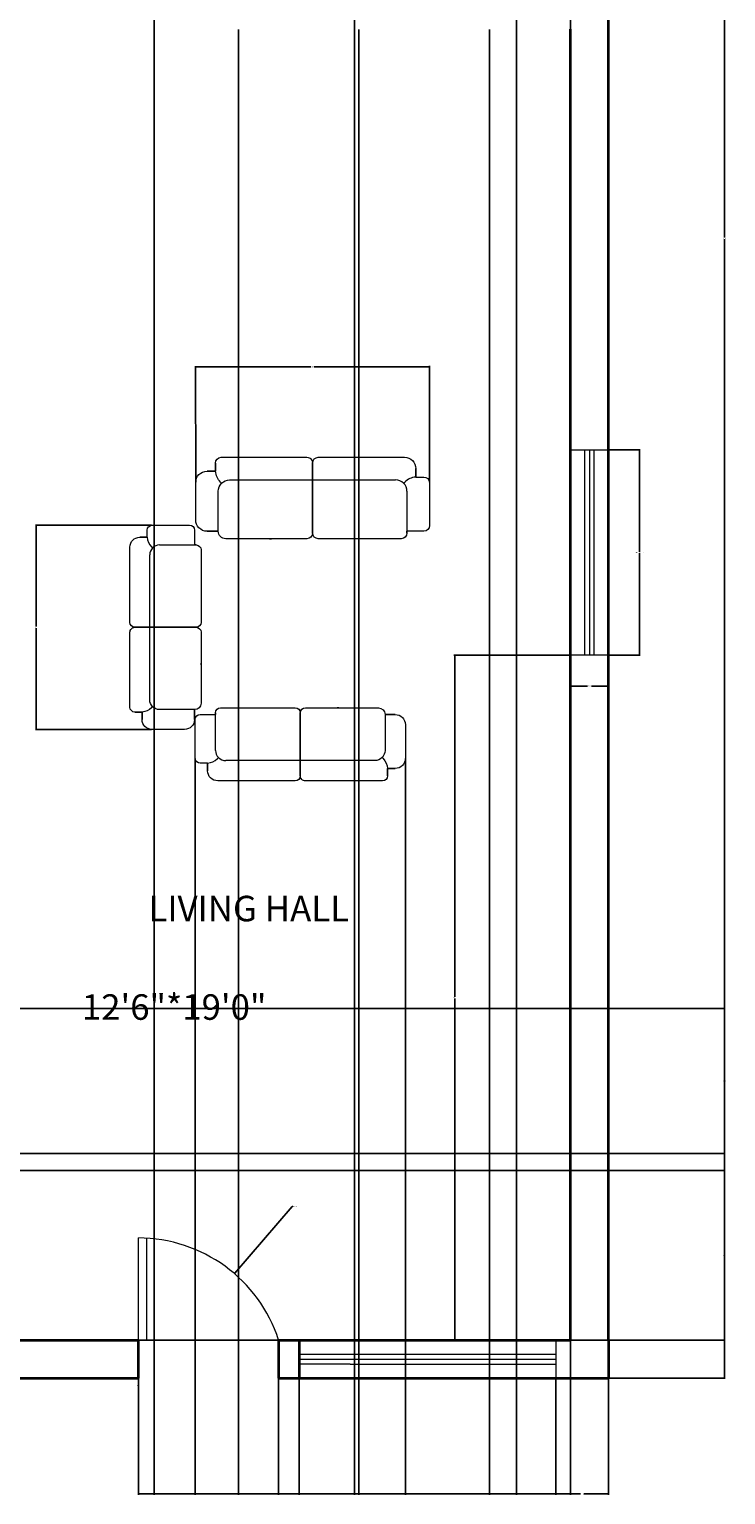
# Model space of a CAD drawing. Units: inches. Extents: x -17 to 1735, y -531 to 60.
# Tile 2 of 27: x 193 to 357, y -531 to -187. Entities that reach past the tile are written whole.
import ezdxf

# ---------------------------------------------------------------- set-up
doc = ezdxf.new("R2010")
doc.units = ezdxf.units.IN
doc.header["$MEASUREMENT"] = 0
for name, color, linetype, lineweight in [('A-ANNO-DIMS', 2, 'Continuous', 18), ('A-AREA-IDEN', 7, 'Continuous', 25), ('A-DOOR', 4, 'Continuous', 18), ('A-GLAZ', 4, 'Continuous', 18), ('A-WALL', 7, 'Continuous', 35)]:
    doc.layers.add(name, color=color, linetype=linetype, lineweight=lineweight)
doc.layers.add('A-FURN', color=242, linetype='Continuous', lineweight=18, true_color=0xcd2027)
doc.styles.get("Standard").update_dxf_attribs({"font": 'arial.ttf'})
doc.dimstyles.get("Standard").update_dxf_attribs({"dimtxt": 0.18, "dimasz": 0.18, "dimexe": 0.18, "dimexo": 0.0625, "dimgap": 0.09, "dimtad": 0, "dimtih": 1, "dimtoh": 1, "dimdec": 4, "dimzin": 0, "dimdsep": 46, "dimtxsty": 'Standard', "dimcen": 0.09, "dimadec": 0, "dimazin": 0, "dimtfac": 1, "dimtdec": 4, "dimtofl": 0, "dimtmove": 0, "dimatfit": 3, "dimfxl": 1, "dimtolj": 1, "dimtzin": 0, "dimarcsym": 0})

# ---------------------------------------------------------------- blocks, each defined once
blk = doc.blocks.new('WIN-FRAME-48IN')
for p, q in [((3.31, 48.33), (3.31, 0)), ((5.59, 0), (5.59, 48.33))]:
    blk.add_line(p, q)
blk.add_lwpolyline([(0, 48.33), (9, 48.33), (9, 0), (0, 0)], close=True)
blk = doc.blocks.new('*D5')
at = {"layer": 'A-ANNO-DIMS', "color": 0, "lineweight": -2, "transparency": 16777216}
for p, q in [((329.12, -285.68), (336.49, -285.68)), ((336.31, -285.86), (336.31, -309.66)), ((336.31, -333.83), (336.31, -310.03)), ((329.12, -334.01), (336.49, -334.01))]:
    blk.add_line(p, q, dxfattribs=at)
at = {"layer": 'A-ANNO-DIMS', "color": 0, "transparency": 16777216}
for points in [[(336.28, -285.86), (336.34, -285.86), (336.31, -285.68)], [(336.28, -333.83), (336.34, -333.83), (336.31, -334.01)]]:
    blk.add_solid(points, dxfattribs=at)
at = {"layer": 'Defpoints', "color": 0, "transparency": 16777216}
for p in [(329.06, -285.68), (336.31, -285.68), (329.06, -334.01)]:
    blk.add_point(p, dxfattribs=at)
at = {"layer": 'A-ANNO-DIMS', "color": 0, "transparency": 16777216, "insert": (336.31, -309.85), "char_height": 0.18, "attachment_point": 5}
blk.add_mtext('\\A1;WINDOW 48 TYP.', dxfattribs=at)
blk = doc.blocks.new('*D6')
at = {"layer": 'A-ANNO-DIMS', "color": 0, "lineweight": -2, "transparency": 16777216}
for p, q in [((320.06, -334.07), (320.06, -341.44)), ((329.06, -334.07), (329.06, -341.44)), ((320.24, -341.26), (324.1, -341.26)), ((328.88, -341.26), (325.02, -341.26))]:
    blk.add_line(p, q, dxfattribs=at)
at = {"layer": 'A-ANNO-DIMS', "color": 0, "transparency": 16777216}
for points in [[(320.24, -341.23), (320.24, -341.29), (320.06, -341.26)], [(328.88, -341.23), (328.88, -341.29), (329.06, -341.26)]]:
    blk.add_solid(points, dxfattribs=at)
at = {"layer": 'Defpoints', "color": 0, "transparency": 16777216}
for p in [(320.06, -334.01), (329.06, -334.01), (329.06, -341.26)]:
    blk.add_point(p, dxfattribs=at)
at = {"layer": 'A-ANNO-DIMS', "color": 0, "transparency": 16777216, "insert": (324.56, -341.26), "char_height": 0.18, "attachment_point": 5}
blk.add_mtext('\\A1;9 TYP.', dxfattribs=at)
blk = doc.blocks.new('*D10')
at = {"layer": 'A-ANNO-DIMS', "color": 0, "lineweight": -2, "transparency": 16777216}
for p, q in [((329.12, 32.23), (356.44, 32.23)), ((356.26, 32.05), (356.26, -235.74)), ((356.26, -503.9), (356.26, -236.11)), ((329.12, -504.08), (356.44, -504.08))]:
    blk.add_line(p, q, dxfattribs=at)
at = {"layer": 'A-ANNO-DIMS', "color": 0, "transparency": 16777216}
for points in [[(356.23, 32.05), (356.29, 32.05), (356.26, 32.23)], [(356.23, -503.9), (356.29, -503.9), (356.26, -504.08)]]:
    blk.add_solid(points, dxfattribs=at)
at = {"layer": 'Defpoints', "color": 0, "transparency": 16777216}
for p in [(329.06, 32.23), (329.06, -504.08), (356.26, -504.08)]:
    blk.add_point(p, dxfattribs=at)
at = {"layer": 'A-ANNO-DIMS', "color": 0, "transparency": 16777216, "insert": (356.26, -235.92), "char_height": 0.18, "attachment_point": 5}
blk.add_mtext('\\A1;536.3', dxfattribs=at)
blk = doc.blocks.new('*D12')
at = {"layer": 'A-ANNO-DIMS', "color": 0, "lineweight": -2, "transparency": 16777216}
for p, q in [((269.33, 23.18), (269.33, -531.46)), ((320.06, 23.17), (320.06, -531.46)), ((269.51, -531.28), (294.3, -531.28)), ((319.88, -531.28), (295.09, -531.28))]:
    blk.add_line(p, q, dxfattribs=at)
at = {"layer": 'A-ANNO-DIMS', "color": 0, "transparency": 16777216}
for points in [[(269.51, -531.25), (269.51, -531.31), (269.33, -531.28)], [(319.88, -531.25), (319.88, -531.31), (320.06, -531.28)]]:
    blk.add_solid(points, dxfattribs=at)
at = {"layer": 'Defpoints', "color": 0, "transparency": 16777216}
for p in [(269.33, 23.24), (320.06, 23.23), (320.06, -531.28)]:
    blk.add_point(p, dxfattribs=at)
at = {"layer": 'A-ANNO-DIMS', "color": 0, "transparency": 16777216, "insert": (294.7, -531.28), "char_height": 0.18, "attachment_point": 5}
blk.add_mtext('\\A1;50.73', dxfattribs=at)
blk = doc.blocks.new('*D20')
at = {"layer": 'A-ANNO-DIMS', "color": 0, "lineweight": -2, "transparency": 16777216}
for p, q in [((320, -334.01), (292.68, -334.01)), ((292.86, -334.19), (292.86, -414.36)), ((292.86, -494.9), (292.86, -414.73)), ((320, -495.08), (292.68, -495.08))]:
    blk.add_line(p, q, dxfattribs=at)
at = {"layer": 'A-ANNO-DIMS', "color": 0, "transparency": 16777216}
for points in [[(292.83, -334.19), (292.89, -334.19), (292.86, -334.01)], [(292.83, -494.9), (292.89, -494.9), (292.86, -495.08)]]:
    blk.add_solid(points, dxfattribs=at)
at = {"layer": 'Defpoints', "color": 0, "transparency": 16777216}
for p in [(292.86, -334.01), (320.06, -334.01), (320.06, -495.08)]:
    blk.add_point(p, dxfattribs=at)
at = {"layer": 'A-ANNO-DIMS', "color": 0, "transparency": 16777216, "insert": (292.86, -414.54), "char_height": 0.18, "attachment_point": 5}
blk.add_mtext('\\A1;161.07', dxfattribs=at)
blk = doc.blocks.new('*D21')
at = {"layer": 'A-ANNO-DIMS', "color": 0, "lineweight": -2, "transparency": 16777216}
for p, q in [((218.5, -504.14), (218.5, -531.46)), ((251.48, -504.14), (251.48, -531.46)), ((218.68, -531.28), (234.59, -531.28)), ((251.3, -531.28), (235.38, -531.28))]:
    blk.add_line(p, q, dxfattribs=at)
at = {"layer": 'A-ANNO-DIMS', "color": 0, "transparency": 16777216}
for points in [[(218.68, -531.25), (218.68, -531.31), (218.5, -531.28)], [(251.3, -531.25), (251.3, -531.31), (251.48, -531.28)]]:
    blk.add_solid(points, dxfattribs=at)
at = {"layer": 'Defpoints', "color": 0, "transparency": 16777216}
for p in [(218.5, -504.08), (251.48, -504.08), (251.48, -531.28)]:
    blk.add_point(p, dxfattribs=at)
at = {"layer": 'A-ANNO-DIMS', "color": 0, "transparency": 16777216, "insert": (234.99, -531.28), "char_height": 0.18, "attachment_point": 5}
blk.add_mtext('\\A1;32.98', dxfattribs=at)
blk = doc.blocks.new('*D22')
at = {"layer": 'A-ANNO-DIMS', "color": 0, "lineweight": -2, "transparency": 16777216}
for p, q in [((251.48, -504.14), (251.48, -531.46)), ((256.31, -504.14), (256.31, -531.46)), ((251.66, -531.28), (253.5, -531.28)), ((256.13, -531.28), (254.29, -531.28))]:
    blk.add_line(p, q, dxfattribs=at)
at = {"layer": 'A-ANNO-DIMS', "color": 0, "transparency": 16777216}
for points in [[(251.66, -531.25), (251.66, -531.31), (251.48, -531.28)], [(256.13, -531.25), (256.13, -531.31), (256.31, -531.28)]]:
    blk.add_solid(points, dxfattribs=at)
at = {"layer": 'Defpoints', "color": 0, "transparency": 16777216}
for p in [(251.48, -504.08), (256.31, -504.08), (256.31, -531.28)]:
    blk.add_point(p, dxfattribs=at)
at = {"layer": 'A-ANNO-DIMS', "color": 0, "transparency": 16777216, "insert": (253.9, -531.28), "char_height": 0.18, "attachment_point": 5}
blk.add_mtext('\\A1;4.837', dxfattribs=at)
blk = doc.blocks.new('*D23')
at = {"layer": 'A-ANNO-DIMS', "color": 0, "lineweight": -2, "transparency": 16777216}
for p, q in [((256.31, -504.14), (256.31, -531.46)), ((316.64, -504.14), (316.64, -531.46)), ((256.49, -531.28), (286.08, -531.28)), ((316.46, -531.28), (286.87, -531.28))]:
    blk.add_line(p, q, dxfattribs=at)
at = {"layer": 'A-ANNO-DIMS', "color": 0, "transparency": 16777216}
for points in [[(256.49, -531.25), (256.49, -531.31), (256.31, -531.28)], [(316.46, -531.25), (316.46, -531.31), (316.64, -531.28)]]:
    blk.add_solid(points, dxfattribs=at)
at = {"layer": 'Defpoints', "color": 0, "transparency": 16777216}
for p in [(256.31, -504.08), (316.64, -504.08), (316.64, -531.28)]:
    blk.add_point(p, dxfattribs=at)
at = {"layer": 'A-ANNO-DIMS', "color": 0, "transparency": 16777216, "insert": (286.48, -531.28), "char_height": 0.18, "attachment_point": 5}
blk.add_mtext('\\A1;60.33', dxfattribs=at)
blk = doc.blocks.new('*D24')
at = {"layer": 'A-ANNO-DIMS', "color": 0, "lineweight": -2, "transparency": 16777216}
for p, q in [((316.64, -504.14), (316.64, -531.46)), ((329.06, -504.14), (329.06, -531.46)), ((316.82, -531.28), (322.47, -531.28)), ((328.88, -531.28), (323.24, -531.28))]:
    blk.add_line(p, q, dxfattribs=at)
at = {"layer": 'A-ANNO-DIMS', "color": 0, "transparency": 16777216}
for points in [[(316.82, -531.25), (316.82, -531.31), (316.64, -531.28)], [(328.88, -531.25), (328.88, -531.31), (329.06, -531.28)]]:
    blk.add_solid(points, dxfattribs=at)
at = {"layer": 'Defpoints', "color": 0, "transparency": 16777216}
for p in [(316.64, -504.08), (329.06, -504.08), (329.06, -531.28)]:
    blk.add_point(p, dxfattribs=at)
at = {"layer": 'A-ANNO-DIMS', "color": 0, "transparency": 16777216, "insert": (322.85, -531.28), "char_height": 0.18, "attachment_point": 5}
blk.add_mtext('\\A1;12.42', dxfattribs=at)
blk = doc.blocks.new('*D27')
at = {"layer": 'A-ANNO-DIMS', "color": 0, "lineweight": -2, "transparency": 16777216}
for p, q in [((242.06, -186.83), (242.06, -531.46)), ((270.3, -186.83), (270.3, -531.46)), ((242.24, -531.28), (255.71, -531.28)), ((270.12, -531.28), (256.65, -531.28))]:
    blk.add_line(p, q, dxfattribs=at)
at = {"layer": 'A-ANNO-DIMS', "color": 0, "transparency": 16777216}
for points in [[(242.24, -531.25), (242.24, -531.31), (242.06, -531.28)], [(270.12, -531.25), (270.12, -531.31), (270.3, -531.28)]]:
    blk.add_solid(points, dxfattribs=at)
at = {"layer": 'Defpoints', "color": 0, "transparency": 16777216}
for p in [(242.06, -186.77), (270.3, -186.77), (270.3, -531.28)]:
    blk.add_point(p, dxfattribs=at)
at = {"layer": 'A-ANNO-DIMS', "color": 0, "transparency": 16777216, "insert": (256.18, -531.28), "char_height": 0.18, "attachment_point": 5}
blk.add_mtext('\\A1;28.237', dxfattribs=at)
blk = doc.blocks.new('*D28')
at = {"layer": 'A-ANNO-DIMS', "color": 0, "lineweight": -2, "transparency": 16777216}
for p, q in [((270.3, -186.83), (270.3, -531.46)), ((301.08, -186.83), (301.08, -531.46)), ((270.48, -531.28), (285.29, -531.28)), ((300.9, -531.28), (286.08, -531.28))]:
    blk.add_line(p, q, dxfattribs=at)
at = {"layer": 'A-ANNO-DIMS', "color": 0, "transparency": 16777216}
for points in [[(270.48, -531.25), (270.48, -531.31), (270.3, -531.28)], [(300.9, -531.25), (300.9, -531.31), (301.08, -531.28)]]:
    blk.add_solid(points, dxfattribs=at)
at = {"layer": 'Defpoints', "color": 0, "transparency": 16777216}
for p in [(270.3, -186.77), (301.08, -186.77), (301.08, -531.28)]:
    blk.add_point(p, dxfattribs=at)
at = {"layer": 'A-ANNO-DIMS', "color": 0, "transparency": 16777216, "insert": (285.69, -531.28), "char_height": 0.18, "attachment_point": 5}
blk.add_mtext('\\A1;30.78', dxfattribs=at)
blk = doc.blocks.new('*D37')
at = {"layer": 'A-ANNO-DIMS', "color": 0, "lineweight": -2, "transparency": 16777216}
for p, q in [((222.24, -32.84), (222.24, -531.46)), ((307.4, -32.94), (307.4, -531.46)), ((222.42, -531.28), (264.43, -531.28)), ((307.22, -531.28), (265.21, -531.28))]:
    blk.add_line(p, q, dxfattribs=at)
at = {"layer": 'A-ANNO-DIMS', "color": 0, "transparency": 16777216}
for points in [[(222.42, -531.25), (222.42, -531.31), (222.24, -531.28)], [(307.22, -531.25), (307.22, -531.31), (307.4, -531.28)]]:
    blk.add_solid(points, dxfattribs=at)
at = {"layer": 'Defpoints', "color": 0, "transparency": 16777216}
for p in [(222.24, -32.78), (307.4, -32.88), (307.4, -531.28)]:
    blk.add_point(p, dxfattribs=at)
at = {"layer": 'A-ANNO-DIMS', "color": 0, "transparency": 16777216, "insert": (264.82, -531.28), "char_height": 0.18, "attachment_point": 5}
blk.add_mtext('\\A1;85.16', dxfattribs=at)
blk = doc.blocks.new('*D39')
at = {"layer": 'A-ANNO-DIMS', "color": 0, "lineweight": -2, "transparency": 16777216}
for p, q in [((231.98, -293.31), (231.97, -265.99)), ((232.15, -266.17), (259.06, -266.16)), ((286.76, -266.14), (259.85, -266.16)), ((286.95, -293.28), (286.94, -265.96))]:
    blk.add_line(p, q, dxfattribs=at)
at = {"layer": 'A-ANNO-DIMS', "color": 0, "transparency": 16777216}
for points in [[(232.15, -266.14), (232.15, -266.2), (231.97, -266.17)], [(286.76, -266.11), (286.76, -266.17), (286.94, -266.14)]]:
    blk.add_solid(points, dxfattribs=at)
at = {"layer": 'Defpoints', "color": 0, "transparency": 16777216}
for p in [(286.94, -266.14), (231.98, -293.37), (286.95, -293.34)]:
    blk.add_point(p, dxfattribs=at)
at = {"layer": 'A-ANNO-DIMS', "color": 0, "transparency": 16777216, "insert": (259.45, -266.16), "char_height": 0.18, "attachment_point": 5}
blk.add_mtext('\\A1;54.97', dxfattribs=at)
blk = doc.blocks.new('*D40')
at = {"layer": 'A-ANNO-DIMS', "color": 0, "lineweight": -2, "transparency": 16777216}
for p, q in [((231.86, -358.31), (231.86, -531.46)), ((281.27, -358.31), (281.27, -531.46)), ((232.04, -531.28), (256.17, -531.28)), ((281.09, -531.28), (256.96, -531.28))]:
    blk.add_line(p, q, dxfattribs=at)
at = {"layer": 'A-ANNO-DIMS', "color": 0, "transparency": 16777216}
for points in [[(232.04, -531.25), (232.04, -531.31), (231.86, -531.28)], [(281.09, -531.25), (281.09, -531.31), (281.27, -531.28)]]:
    blk.add_solid(points, dxfattribs=at)
at = {"layer": 'Defpoints', "color": 0, "transparency": 16777216}
for p in [(231.86, -358.25), (281.27, -358.25), (281.27, -531.28)]:
    blk.add_point(p, dxfattribs=at)
at = {"layer": 'A-ANNO-DIMS', "color": 0, "transparency": 16777216, "insert": (256.56, -531.28), "char_height": 0.18, "attachment_point": 5}
blk.add_mtext('\\A1;49.42', dxfattribs=at)
blk = doc.blocks.new('*D41')
at = {"layer": 'A-ANNO-DIMS', "color": 0, "lineweight": -2, "transparency": 16777216}
for p, q in [((221.6, -303.41), (194.29, -303.43)), ((194.47, -303.61), (194.48, -327.26)), ((194.49, -351.27), (194.48, -327.62)), ((221.63, -351.44), (194.31, -351.45))]:
    blk.add_line(p, q, dxfattribs=at)
at = {"layer": 'A-ANNO-DIMS', "color": 0, "transparency": 16777216}
for points in [[(194.5, -303.61), (194.44, -303.61), (194.47, -303.43)], [(194.52, -351.27), (194.46, -351.27), (194.49, -351.45)]]:
    blk.add_solid(points, dxfattribs=at)
at = {"layer": 'Defpoints', "color": 0, "transparency": 16777216}
for p in [(194.47, -303.43), (221.67, -303.41), (221.69, -351.44)]:
    blk.add_point(p, dxfattribs=at)
at = {"layer": 'A-ANNO-DIMS', "color": 0, "transparency": 16777216, "insert": (194.48, -327.44), "char_height": 0.18, "attachment_point": 5}
blk.add_mtext('\\A1;48.03', dxfattribs=at)
blk = doc.blocks.new('*D51')
at = {"layer": 'A-ANNO-DIMS', "color": 0, "lineweight": -2, "transparency": 16777216}
for p, q in [((152.12, -417.08), (356.44, -417.08)), ((356.26, -417.26), (356.26, -433.97)), ((356.26, -451.04), (356.26, -434.33)), ((152.12, -451.22), (356.44, -451.22))]:
    blk.add_line(p, q, dxfattribs=at)
at = {"layer": 'A-ANNO-DIMS', "color": 0, "transparency": 16777216}
for points in [[(356.23, -417.26), (356.29, -417.26), (356.26, -417.08)], [(356.23, -451.04), (356.29, -451.04), (356.26, -451.22)]]:
    blk.add_solid(points, dxfattribs=at)
at = {"layer": 'Defpoints', "color": 0, "transparency": 16777216}
for p in [(152.06, -417.08), (152.06, -451.22), (356.26, -451.22)]:
    blk.add_point(p, dxfattribs=at)
at = {"layer": 'A-ANNO-DIMS', "color": 0, "transparency": 16777216, "insert": (356.26, -434.15), "char_height": 0.18, "attachment_point": 5}
blk.add_mtext('\\A1;34.14', dxfattribs=at)
blk = doc.blocks.new('*D52')
at = {"layer": 'A-ANNO-DIMS', "color": 0, "lineweight": -2, "transparency": 16777216}
for p, q in [((162.53, -455.22), (356.44, -455.22)), ((356.26, -455.4), (356.26, -474.97)), ((356.26, -494.9), (356.26, -475.33)), ((162.53, -495.08), (356.44, -495.08))]:
    blk.add_line(p, q, dxfattribs=at)
at = {"layer": 'A-ANNO-DIMS', "color": 0, "transparency": 16777216}
for points in [[(356.23, -455.4), (356.29, -455.4), (356.26, -455.22)], [(356.23, -494.9), (356.29, -494.9), (356.26, -495.08)]]:
    blk.add_solid(points, dxfattribs=at)
at = {"layer": 'Defpoints', "color": 0, "transparency": 16777216}
for p in [(162.47, -455.22), (162.47, -495.08), (356.26, -495.08)]:
    blk.add_point(p, dxfattribs=at)
at = {"layer": 'A-ANNO-DIMS', "color": 0, "transparency": 16777216, "insert": (356.26, -475.15), "char_height": 0.18, "attachment_point": 5}
blk.add_mtext('\\A1;39.86', dxfattribs=at)
blk = doc.blocks.new('*D58')
at = {"layer": 'A-ANNO-DIMS', "color": 0, "lineweight": -2, "transparency": 16777216}
for p, q in [((254.66, -463.67), (241.2, -479.33)), ((254.84, -463.67), (254.66, -463.67)), ((218.37, -505.8), (218.55, -505.8)), ((218.46, -505.89), (218.46, -505.71))]:
    blk.add_line(p, q, dxfattribs=at)
at = {"layer": 'A-ANNO-DIMS', "color": 0, "transparency": 16777216}
blk.add_solid([(241.18, -479.31), (241.22, -479.35), (241.08, -479.47)], dxfattribs=at)
at = {"layer": 'Defpoints', "color": 0, "transparency": 16777216}
for p in [(241.08, -479.47), (218.46, -505.8)]:
    blk.add_point(p, dxfattribs=at)
at = {"layer": 'A-ANNO-DIMS', "color": 0, "transparency": 16777216, "insert": (255.32, -463.67), "char_height": 0.18, "attachment_point": 5}
blk.add_mtext('\\A1;R34.72', dxfattribs=at)

msp = doc.modelspace()

# ---------------------------------------------------------------- linework, layer by layer
at = {"layer": 'A-DOOR'}
for p, q in [((218.4964, -495.0795), (218.4964, -471.0795)), ((220.4964, -495.0795), (220.4964, -471.1395)), ((220.4964, -495.0795), (218.4964, -495.0795))]:
    msp.add_line(p, q, dxfattribs=at)
msp.add_arc((218.4553, -505.7987), 34.7192, 17.98326, 89.932167, dxfattribs=at)
at = {"layer": 'A-FURN'}
for p, q in [((236.6372, -288.7839), (236.6372, -290.7077)), ((259.4662, -288.7751), (259.4662, -305.2679)), ((259.4662, -305.2679), (259.4662, -288.7751)), ((236.6449, -290.7077), (234.6383, -290.7077)), ((239.9586, -292.7741), (259.4662, -292.7653)), ((259.4662, -292.7653), (278.9738, -292.7653)), ((283.7004, -292.1118), (283.7004, -290.1052)), ((237.2984, -304.8321), (237.2984, -295.4343)), ((238.0776, -293.5533), (237.8059, -293.2816)), ((280.8548, -293.5444), (281.1265, -293.2728)), ((281.634, -295.4254), (281.634, -304.8321)), ((220.5916, -306.2544), (218.8386, -306.2544)), ((234.6383, -304.8321), (237.2984, -304.8321)), ((249.3652, -306.598), (249.801, -306.598)), ((281.634, -305.2679), (281.634, -304.8321)), ((221.8433, -308.7404), (221.6059, -308.5031)), ((223.4866, -308.0597), (231.7047, -308.0597)), ((232.0855, -308.0597), (231.7047, -308.0597)), ((221.1626, -327.4265), (221.1626, -310.3837)), ((217.6766, -327.4265), (232.0855, -327.4265)), ((232.0855, -327.4265), (217.6766, -327.4265)), ((221.1703, -344.4693), (221.1626, -327.4265)), ((233.2475, -336.2512), (233.2475, -335.8705)), ((217.6843, -347.371), (219.365, -347.371)), ((219.365, -347.3643), (219.365, -349.1173)), ((221.851, -346.1126), (221.6137, -346.35)), ((231.7047, -346.7933), (223.4943, -346.7933)), ((231.7047, -349.1173), (231.7047, -346.7933)), ((236.6379, -356.3791), (236.642, -347.9235)), ((236.6421, -347.5317), (236.642, -347.9235)), ((256.5616, -362.3667), (256.5688, -347.5413)), ((256.5688, -347.5413), (256.5616, -362.3667)), ((265.6491, -346.3501), (265.2573, -346.3499)), ((276.4952, -347.9428), (276.4911, -356.3904)), ((278.8864, -347.9439), (276.4952, -347.9428)), ((237.3374, -358.0703), (237.0931, -358.3144)), ((275.7899, -358.0809), (276.034, -358.3252)), ((234.7789, -359.3569), (234.778, -361.1606)), ((256.5633, -358.7799), (239.0279, -358.7715)), ((274.0987, -358.7805), (256.5633, -358.7799)), ((277.0765, -360.6394), (278.8802, -360.6403)), ((277.0826, -362.3687), (277.0834, -360.6394))]:
    msp.add_line(p, q, dxfattribs=at)
for points in [[(280.3039, -306.598), (260.7963, -306.598, -0.41421356), (259.4662, -305.2679, -0.41421356), (258.1361, -306.598), (249.801, -306.598), (249.801, -306.598, -0.41421356), (249.801, -306.598), (239.037, -306.598, -0.40429871), (237.2984, -304.8321), (234.6383, -304.8321, -0.41421356), (231.9781, -302.1719), (231.9781, -293.3679, -0.41421356), (234.6383, -290.7077), (236.6372, -290.7077), (236.6372, -288.7839, -0.40953287), (237.9673, -287.445), (258.1361, -287.445, -0.4144824), (259.4662, -288.7751, -0.41421356), (260.7963, -287.445), (281.0403, -287.445, -0.41421356), (283.7004, -290.1052), (283.7004, -292.1041), (285.6242, -292.1041, -0.39431507), (286.9511, -293.3432), (286.9542, -303.502, -0.41421005), (285.6242, -304.8321), (281.634, -304.8321), (281.634, -305.2679, -0.41421356), (280.3039, -306.598, -2.41421356)], [(233.2475, -309.2217), (233.2475, -326.2645, -0.41421356), (232.0855, -327.4265, -0.41421356), (233.2475, -328.5885), (233.2475, -335.8705), (233.2475, -335.8705, -0.41421356), (233.2475, -335.8705), (233.2475, -345.2744, -0.40429871), (231.7047, -346.7933), (231.7047, -349.1173, -0.41421356), (229.3807, -351.4414), (221.689, -351.4414, -0.41421356), (219.365, -349.1173), (219.365, -347.371), (217.6843, -347.371, -0.40953287), (216.5145, -346.209), (216.5145, -328.5885, -0.4144824), (217.6766, -327.4265, -0.41421356), (216.5145, -326.2645), (216.5145, -308.5784, -0.41421356), (218.8386, -306.2544), (220.5849, -306.2544), (220.5849, -304.5737, -0.39431507), (221.6675, -303.4144), (230.5427, -303.4117, -0.41421005), (231.7047, -304.5737), (231.7047, -308.0597), (232.0855, -308.0597, -0.41421356), (233.2475, -309.2217, -2.41421356)], [(237.8383, -346.3367), (255.3737, -346.3452, -0.41421356), (256.5688, -347.5413, -0.41421356), (257.7649, -346.3463), (265.2573, -346.3499), (265.2573, -346.3499, -0.41421356), (265.2573, -346.3499), (274.9331, -346.3546, -0.40429871), (276.4952, -347.9428), (278.8864, -347.9439, -0.41421356), (281.2764, -350.3363), (281.2726, -358.2503, -0.41421356), (278.8802, -360.6403), (277.0834, -360.6394), (277.0826, -362.3687, -0.40953287), (275.8864, -363.5717), (257.7566, -363.5629, -0.4144824), (256.5616, -362.3667, -0.41421356), (255.3654, -363.5617), (237.1681, -363.5529, -0.41421356), (234.778, -361.1606), (234.7789, -359.3638), (233.0496, -359.3629, -0.39431507), (231.8574, -358.2485), (231.859, -349.1168, -0.41421005), (233.0552, -347.9217), (236.642, -347.9235), (236.6421, -347.5317, -0.41421356), (237.8383, -346.3367, -2.41421356)]]:
    msp.add_lwpolyline(points, format="xyb", dxfattribs=at)
at = {"layer": 'A-FURN', "extrusion": (0, 0, -1)}
for centre, major_axis, start_param, end_param in [((240.6274, -290.4601), (-2.8215, -2.8215), 0, 0.72330723), ((239.9586, -295.4343), (1.881, -1.881), 2.35619449, 3.92699082), ((223.4943, -344.4693), (1.6433, 1.6433), 2.35619449, 3.92699082), ((219.1487, -343.885), (2.465, -2.465), 0, 0.72330723), ((274.0999, -356.3893), (-1.69, 1.6916), 2.35619449, 3.92699082), ((273.4965, -360.8603), (2.5375, 2.535), 0, 0.72330723)]:
    msp.add_ellipse(centre, major_axis=major_axis, ratio=1, start_param=start_param, end_param=end_param, dxfattribs=at)
at = {"layer": 'A-FURN'}
for centre, major_axis, start_param, end_param in [((278.9738, -295.4254), (1.881, -1.881), 0.78539816, 2.35619449), ((283.948, -296.0943), (-2.8215, -2.8215), 3.98908175, 4.71238898), ((224.0709, -306.0381), (2.465, -2.465), 3.98908175, 4.71238898), ((223.4866, -310.3837), (1.6433, 1.6433), 0.78539816, 2.35619449), ((234.5581, -355.7769), (2.5375, 2.535), 3.98908175, 4.71238898), ((239.0291, -356.3803), (-1.69, 1.6916), 0.78539816, 2.35619449)]:
    msp.add_ellipse(centre, major_axis=major_axis, ratio=1, start_param=start_param, end_param=end_param, dxfattribs=at)
at = {"layer": 'A-GLAZ'}
for p, q in [((324.5875, -285.6824), (324.5875, -334.0081)), ((256.315, -504.0795), (256.315, -495.0795)), ((256.315, -495.0795), (268.315, -495.0795)), ((268.315, -498.4867), (256.315, -498.4867)), ((316.6407, -499.6342), (256.315, -499.6342)), ((316.6407, -498.4867), (268.315, -498.4867)), ((268.315, -500.7684), (256.315, -500.7684)), ((268.315, -500.7684), (316.6407, -500.7684)), ((268.315, -504.0795), (256.315, -504.0795))]:
    msp.add_line(p, q, dxfattribs=at)
msp.add_lwpolyline([(268.315, -495.0795), (316.6407, -495.0795), (316.6407, -504.0795), (268.315, -504.0795)], dxfattribs=at)
at = {"layer": 'A-WALL'}
for p, q in [((329.0618, -495.0795), (329.0618, 32.2315)), ((320.0618, -495.0795), (320.0618, -186.7685)), ((20.0618, -495.0795), (218.4964, -495.0795)), ((218.4964, -504.0795), (218.4964, -495.0795)), ((251.4783, -495.0795), (320.0618, -495.0795)), ((251.4783, -495.0795), (251.4783, -504.0795)), ((256.315, -495.0795), (256.315, -504.0795)), ((329.0618, -495.0795), (329.0618, -504.0795)), ((20.0618, -504.0795), (218.4964, -504.0795)), ((251.4783, -504.0795), (329.0618, -504.0795))]:
    msp.add_line(p, q, dxfattribs=at)

# ---------------------------------------------------------------- block references
at = {"layer": 'A-GLAZ'}
msp.add_blockref('WIN-FRAME-48IN', (320.062, -334.008), dxfattribs=at)

# ---------------------------------------------------------------- texts
at = {"layer": 'A-ANNO-DIMS', "insert": (205.221, -413.7529), "char_height": 6, "attachment_point": 1}
msp.add_mtext_dynamic_manual_height_columns('12\'6"*19\'0"', width=118.451087, gutter_width=1, heights=[0], dxfattribs=at)
at = {"layer": 'A-AREA-IDEN', "insert": (220.8794, -390.583), "char_height": 6, "attachment_point": 1}
msp.add_mtext_dynamic_manual_height_columns('LIVING HALL', width=74.275107, gutter_width=1, heights=[0], dxfattribs=at)

# ---------------------------------------------------------------- dimensions: what is measured, and where the dimension line sits
at = {"layer": 'A-ANNO-DIMS'}
for base, p1, p2, angle, override, picture, middle in [((356.2618, -504.0795), (329.0618, 32.2315), (329.0618, -504.0795), 270, {"dimdec": 1, "dimlfac": 1, "dimrnd": 0, "dimzin": 0, "dimdsep": 46, "dimlunit": 2}, '*D10', (356.2618, -235.924)), ((286.9389, -266.1432), (231.9781, -293.3679), (286.9511, -293.3432), 0.025679, {"dimdec": 2, "dimlfac": 1, "dimrnd": 0, "dimzin": 0, "dimdsep": 46, "dimlunit": 2}, '*D39', (259.4525, -266.1555)), ((194.4675, -303.4266), (221.689, -351.4414), (221.6675, -303.4144), 90.025679, {"dimdec": 2, "dimlfac": 1, "dimrnd": 0, "dimzin": 0, "dimdsep": 46, "dimlunit": 2}, '*D41', (194.4782, -327.4401)), ((292.8618, -334.0081), (320.0618, -495.0795), (320.0618, -334.0081), 90, {"dimdec": 2, "dimlfac": 1, "dimrnd": 0, "dimzin": 0, "dimdsep": 46, "dimlunit": 2}, '*D20', (292.8618, -414.5438)), ((356.2618, -451.2168), (152.0618, -417.0795), (152.0618, -451.2168), 90, {"dimdec": 2, "dimlfac": 1, "dimrnd": 0, "dimzin": 0, "dimdsep": 46, "dimlunit": 2}, '*D51', (356.2618, -434.1481)), ((356.2618, -495.0795), (162.4671, -455.2168), (162.4671, -495.0795), 90, {"dimdec": 2, "dimlfac": 1, "dimrnd": 0, "dimzin": 0, "dimdsep": 46, "dimlunit": 2}, '*D52', (356.2618, -475.1481))]:
    dim = msp.add_linear_dim(base=base, p1=p1, p2=p2, angle=angle, dimstyle='Standard', override=override, dxfattribs=at)
    dim.commit()
    dim.dimension.update_dxf_attribs({"geometry": picture, "text_midpoint": middle})
for base, p1, p2, override, picture, middle in [((320.0618, -531.2795), (269.333, 23.2408), (320.0618, 23.2315), {"dimdec": 2, "dimlfac": 1, "dimrnd": 0, "dimzin": 0, "dimdsep": 46, "dimlunit": 2}, '*D12', (294.6974, -531.2795)), ((307.402, -531.2795), (222.238, -32.7807), (307.402, -32.8805), {"dimdec": 2, "dimlfac": 1, "dimrnd": 0, "dimzin": 0, "dimdsep": 46, "dimlunit": 2}, '*D37', (264.82, -531.2795)), ((270.29831, -531.27951), (242.06178, -186.76847), (270.29831, -186.76847), {"dimdec": 3, "dimlfac": 1, "dimrnd": 0, "dimzin": 0, "dimdsep": 46, "dimlunit": 2}, '*D27', (256.18005, -531.27951)), ((301.0793, -531.2795), (270.2983, -186.7685), (301.0793, -186.7685), {"dimdec": 2, "dimlfac": 1, "dimrnd": 0, "dimzin": 0, "dimdsep": 46, "dimlunit": 2}, '*D28', (285.6888, -531.2795)), ((281.2726, -531.2795), (231.8574, -358.2485), (281.2726, -358.2503), {"dimdec": 2, "dimlfac": 1, "dimrnd": 0, "dimzin": 0, "dimdsep": 46, "dimlunit": 2}, '*D40', (256.565, -531.2795)), ((251.4783, -531.2795), (218.4964, -504.0795), (251.4783, -504.0795), {"dimdec": 2, "dimlfac": 1, "dimrnd": 0, "dimzin": 0, "dimdsep": 46, "dimlunit": 2}, '*D21', (234.9873, -531.2795)), ((256.315, -531.2795), (251.4783, -504.0795), (256.315, -504.0795), {"dimdec": 3, "dimlfac": 1, "dimrnd": 0, "dimzin": 0, "dimdsep": 46, "dimlunit": 2}, '*D22', (253.8966, -531.2795)), ((316.6407, -531.2795), (256.315, -504.0795), (316.6407, -504.0795), {"dimdec": 2, "dimlfac": 1, "dimrnd": 0, "dimzin": 0, "dimdsep": 46, "dimlunit": 2}, '*D23', (286.4778, -531.2795)), ((329.0618, -531.2795), (316.6407, -504.0795), (329.0618, -504.0795), {"dimdec": 2, "dimlfac": 1, "dimrnd": 0, "dimzin": 0, "dimdsep": 46, "dimlunit": 2}, '*D24', (322.8513, -531.2795))]:
    dim = msp.add_linear_dim(base=base, p1=p1, p2=p2, dimstyle='Standard', override=override, dxfattribs=at)
    dim.commit()
    dim.dimension.update_dxf_attribs({"geometry": picture, "text_midpoint": middle})
dim = msp.add_linear_dim(base=(336.3106, -285.6824), p1=(329.0618, -334.0081), p2=(329.0618, -285.6824), angle=90, text='WINDOW <> TYP.', dimstyle='Standard', override={"dimdec": 0, "dimlfac": 1, "dimrnd": 0, "dimzin": 0, "dimdsep": 46, "dimlunit": 2}, dxfattribs=at)
dim.commit()
dim.dimension.update_dxf_attribs({"geometry": '*D5', "text_midpoint": (336.3106, -309.8452)})
dim = msp.add_linear_dim(base=(329.0618, -341.257), p1=(320.0618, -334.0081), p2=(329.0618, -334.0081), text='<> TYP.', dimstyle='Standard', override={"dimdec": 0, "dimlfac": 1, "dimrnd": 0, "dimzin": 0, "dimdsep": 46, "dimlunit": 2}, dxfattribs=at)
dim.commit()
dim.dimension.update_dxf_attribs({"geometry": '*D6', "text_midpoint": (324.5618, -341.257)})
dim = msp.add_radius_dim(center=(218.4553, -505.7987), mpoint=(241.0835, -479.4665), dimstyle='Standard', override={"dimdec": 2, "dimlfac": 1, "dimrnd": 0, "dimzin": 0, "dimdsep": 46, "dimlunit": 2}, dxfattribs=at)
dim.commit()
dim.dimension.update_dxf_attribs({"geometry": '*D58', "text_midpoint": (255.3194, -463.6672), "dimtype": 164})

doc.saveas('drawing.dxf')
